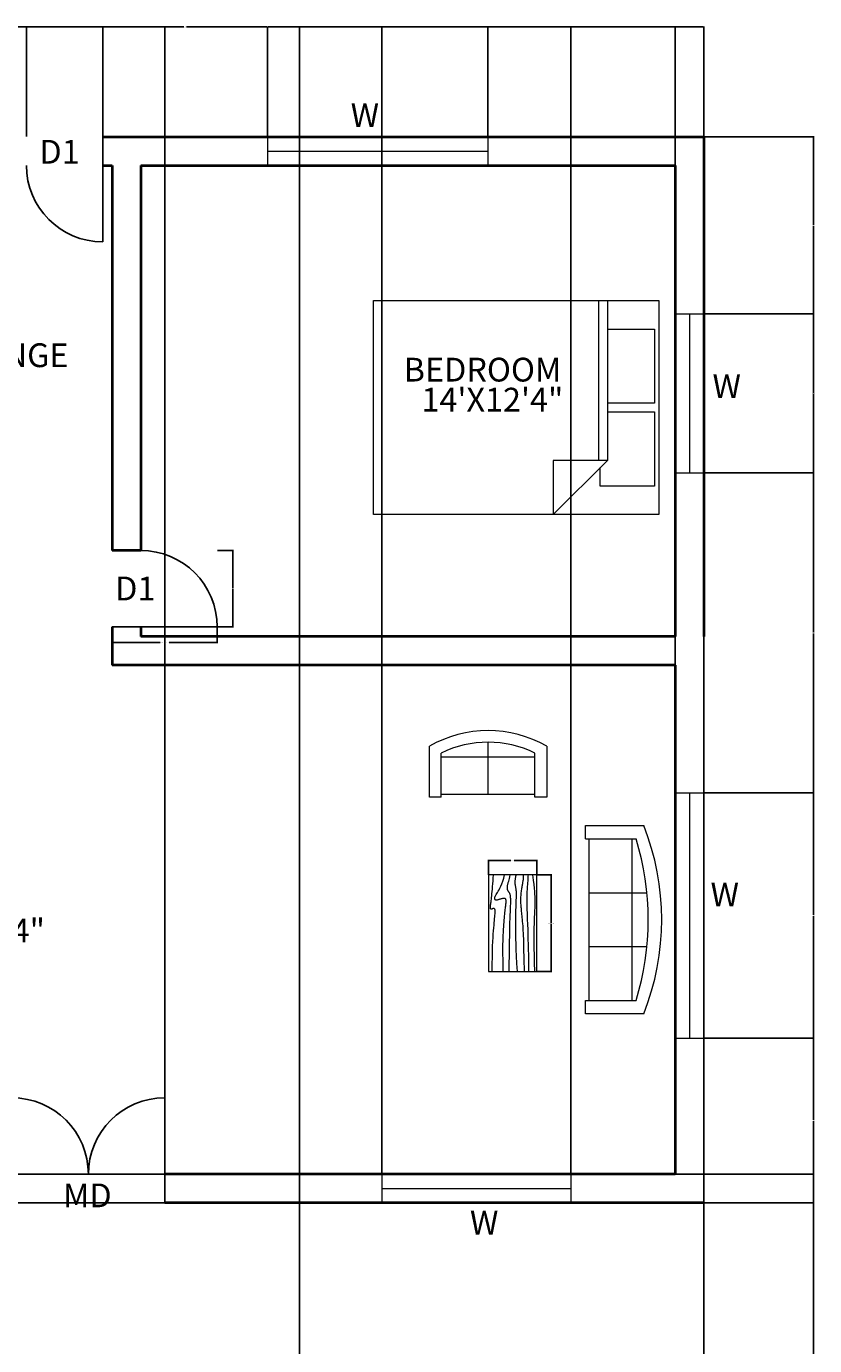
# Model space of a CAD drawing. Units: feet. Extents: x 2032 to 2763, y 1402 to 2145.
# Tile 6 of 6: x 2515 to 2763, y 1731 to 2145. Entities that reach past the tile are written whole.
import ezdxf

# ---------------------------------------------------------------- set-up
doc = ezdxf.new("R2010")
doc.units = ezdxf.units.FT
for name, color, linetype, lineweight in [('A-ANNO-DIMS', 2, 'Continuous', 18), ('A-ANNO-TEXT', 7, 'Continuous', 18), ('A-AREA-IDEN', 7, 'Continuous', 25), ('A-DOOR', 3, 'Continuous', 25), ('A-FLOR', 7, 'Continuous', 25), ('A-FURN', 8, 'Continuous', 18), ('A-GLAZ', 4, 'Continuous', 18), ('A-WALL', 7, 'Continuous', 40), ('C-PROP', 8, 'Continuous', 25)]:
    doc.layers.add(name, color=color, linetype=linetype, lineweight=lineweight)
doc.styles.get("Standard").update_dxf_attribs({"font": 'arial.ttf'})
doc.dimstyles.get("Standard").update_dxf_attribs({"dimtxt": 0.18, "dimasz": 0.18, "dimexe": 0.18, "dimexo": 0.0625, "dimgap": 0.09, "dimtad": 0, "dimtih": 1, "dimtoh": 1, "dimdec": 4, "dimzin": 0, "dimdsep": 46, "dimtxsty": 'Standard', "dimcen": 0.09, "dimadec": 0, "dimazin": 0, "dimtfac": 1, "dimtdec": 4, "dimtofl": 0, "dimtmove": 0, "dimatfit": 3, "dimfxl": 1, "dimtolj": 1, "dimtzin": 0, "dimarcsym": 0})

# ---------------------------------------------------------------- blocks, each defined once
blk = doc.blocks.new('Bed - Queen')
for p, q in [((0, -80.00003), (0, 0)), ((0, 0), (59.99999, 0)), ((59.99999, 0), (59.99999, -80.00003)), ((7.99999, -1.2), (28.79998, -1.2)), ((7.99999, -14.4), (7.99999, -1.2)), ((28.79998, -1.2), (28.79998, -14.4)), ((31.19999, -1.2), (51.99999, -1.2)), ((31.19999, -14.4), (31.19999, -1.2)), ((51.99999, -1.2), (51.99999, -16.4)), ((0, -14.4), (44.8, -14.4)), ((59.99999, -29.6), (44.8, -14.4)), ((44.8, -14.4), (44.8, -29.6)), ((44.8, -16.8), (0, -16.8)), ((51.99999, -16.4), (46.79936, -16.4)), ((44.8, -29.6), (59.99999, -29.6)), ((59.99999, -80.00003), (0, -80.00003))]:
    blk.add_line(p, q)
blk = doc.blocks.new('Sofa - Roundback 7 ft.')
for p, q in [((-36.000027, -34), (-36.000027, -11.4696)), ((-12.00002, -32.4421), (-12.00003, -6.5971)), ((11.99997, -32.4421), (11.99998, -6.5971)), ((35.99998, -34), (35.99998, -11.4696)), ((-35.999844, -13.3819), (35.9998, -13.3819)), ((-36.000027, -32.4421), (35.99998, -32.4421))]:
    blk.add_line(p, q)
for points in [[(-36.000027, -34), (-42.000027, -34), (-42.000027, -8)], [(41.99998, -8), (41.99998, -34), (35.99998, -34)]]:
    blk.add_lwpolyline(points)
for centre, radius, start, end in [((0, -114.25), 114.25, 68.43141, 111.5686), ((-0.00001, -127.1968), 121.1968, 72.72033, 107.2797)]:
    blk.add_arc(centre, radius, start, end)
blk = doc.blocks.new('Sofa - Roundback Loveseat 5 ft.')
for p, q in [((0, -32.44198), (0, -5.99998)), ((-24, -33.99998), (-24, -11.46958)), ((-23.9998, -13.38178), (23.99986, -13.38178)), ((24.00004, -33.99998), (24.00004, -11.46958)), ((-24, -32.44198), (24.00004, -32.44198))]:
    blk.add_line(p, q)
for points in [[(-24, -33.99998), (-30, -33.99998), (-30, -7.99998)], [(30.00004, -7.99998), (30.00004, -33.99998), (24.00004, -33.99998)]]:
    blk.add_lwpolyline(points)
for centre, radius, start, end in [((0, -60.24998), 60.24998, 60.13715, 119.8628), ((0, -61.38438), 55.38444, 64.32083, 115.6792)]:
    blk.add_arc(centre, radius, start, end)
blk = doc.blocks.new('Table - Rectangular Woodgrain 60 x 30 in.')
for p, q in [((0, 0), (0, -30)), ((60, 0), (0, 0)), ((60, -30), (60, 0)), ((0, -30), (60, -30))]:
    blk.add_line(p, q)
for points in [[(0, -2.4), (4.8155, -2.418), (9.0302, -2.4688), (12.709, -2.5477), (15.9167, -2.65), (18.7181, -2.7711), (21.1781, -2.9063), (23.3616, -3.0508), (25.3333, -3.2), (27.1477, -3.3495), (28.8172, -3.4958), (30.3437, -3.636), (31.7291, -3.7667), (32.9756, -3.8849), (34.0849, -3.9875), (35.059, -4.0714), (35.9, -4.1334), (36.6114, -4.1711), (37.2041, -4.1854), (37.6906, -4.1779), (38.0833, -4.15), (38.3948, -4.1034), (38.6375, -4.0396), (38.8239, -3.9602), (38.9666, -3.8667), (39.0764, -3.7608), (39.1573, -3.6448), (39.2116, -3.521), (39.2416, -3.3917), (39.2498, -3.2593), (39.2385, -3.1261), (39.21, -2.9944), (39.1666, -2.8667), (39.111, -2.7447), (39.0468, -2.6281), (38.978, -2.5163), (38.9083, -2.4083), (38.8418, -2.3035), (38.7823, -2.201), (38.7337, -2.1001), (38.7, -2), (38.6844, -1.9003), (38.6875, -1.8021), (38.7094, -1.707), (38.75, -1.6167), (38.8094, -1.5326), (38.8875, -1.4563), (38.9844, -1.3893), (39.1, -1.3333), (39.2351, -1.2896), (39.3937, -1.2583), (39.5804, -1.2396), (39.8, -1.2333), (40.057, -1.2396), (40.3562, -1.2583), (40.7023, -1.2896), (41.1, -1.3333), (41.5547, -1.3895), (42.0755, -1.4573), (42.6721, -1.5361), (43.3542, -1.625), (44.1316, -1.7233), (45.014, -1.8302), (46.0114, -1.9449), (47.1333, -2.0667), (48.3862, -2.1947), (49.7625, -2.3281), (51.2513, -2.4663), (52.8416, -2.6083), (54.5226, -2.7535), (56.2833, -2.9011), (58.1127, -3.0501), (60, -3.2)], [(0, -9.2), (6.5759, -9.0858), (11.9385, -9.0365), (16.2527, -9.0418), (19.6833, -9.0917), (22.3952, -9.1759), (24.5531, -9.2844), (26.322, -9.4069), (27.8666, -9.5333), (29.3241, -9.6553), (30.7203, -9.7719), (32.0532, -9.8837), (33.3208, -9.9917), (34.5213, -10.0965), (35.6526, -10.199), (36.7128, -10.2999), (37.7, -10.4), (38.6129, -10.4996), (39.4531, -10.5969), (40.223, -10.6895), (40.925, -10.775), (41.5613, -10.8512), (42.1344, -10.9156), (42.6465, -10.966), (43.1, -11), (43.4976, -11.0158), (43.8437, -11.0136), (44.143, -10.9942), (44.4, -10.9583), (44.6195, -10.9069), (44.8062, -10.8406), (44.9648, -10.7603), (45.1, -10.6667), (45.2155, -10.5598), (45.3114, -10.4365), (45.3871, -10.2929), (45.4416, -10.125), (45.4743, -9.929), (45.4844, -9.7011), (45.4709, -9.4371), (45.4333, -9.1333), (45.3716, -8.7883), (45.2896, -8.4104), (45.1919, -8.0107), (45.0833, -7.6), (44.9685, -7.1893), (44.8521, -6.7896), (44.7388, -6.4117), (44.6333, -6.0667), (44.54, -5.7628), (44.4614, -5.4979), (44.4001, -5.2675), (44.3583, -5.0667), (44.3384, -4.8909), (44.3427, -4.7354), (44.3736, -4.5956), (44.4333, -4.4667), (44.5236, -4.3453), (44.6427, -4.2333), (44.7884, -4.1339), (44.9583, -4.05), (45.1501, -3.9849), (45.3614, -3.9417), (45.59, -3.9234), (45.8333, -3.9333), (46.0915, -3.9749), (46.3734, -4.0531), (46.6906, -4.1736), (47.0542, -4.3417), (47.4756, -4.5629), (47.9661, -4.8427), (48.5372, -5.1866), (49.2, -5.6), (49.9676, -6.0844), (50.8594, -6.625), (51.8965, -7.2031), (53.1, -7.8), (54.491, -8.3969), (56.0906, -8.975), (57.9199, -9.5156), (60, -10)], [(0, -12.8), (5.1847, -12.9322), (9.6213, -13.0323), (13.3963, -13.1059), (16.5958, -13.1583), (19.3063, -13.1952), (21.614, -13.2219), (23.6054, -13.2439), (25.3666, -13.2667), (26.9728, -13.2947), (28.4531, -13.3281), (29.8256, -13.3663), (31.1083, -13.4083), (32.3191, -13.4535), (33.476, -13.501), (34.597, -13.5501), (35.7, -13.6), (36.7984, -13.6497), (37.8875, -13.6979), (38.9578, -13.743), (40, -13.7833), (41.0047, -13.8174), (41.9625, -13.8438), (42.864, -13.8607), (43.7, -13.8667), (44.4631, -13.8604), (45.1552, -13.8417), (45.7801, -13.8104), (46.3416, -13.7667), (46.8439, -13.7104), (47.2906, -13.6417), (47.6858, -13.5604), (48.0333, -13.4667), (48.3375, -13.3608), (48.6042, -13.2448), (48.8396, -13.121), (49.05, -12.9917), (49.2417, -12.8593), (49.4208, -12.7261), (49.5937, -12.5944), (49.7667, -12.4667), (49.9452, -12.3451), (50.1323, -12.2313), (50.3303, -12.1268), (50.5416, -12.0333), (50.7686, -11.9524), (51.0135, -11.8854), (51.2788, -11.8341), (51.5666, -11.8), (51.8785, -11.7843), (52.2116, -11.7865), (52.562, -11.8059), (52.926, -11.8417), (53.2998, -11.8931), (53.6795, -11.9594), (54.0614, -12.0397), (54.4416, -12.1333), (54.8223, -12.2401), (55.2293, -12.3625), (55.6942, -12.5037), (56.2489, -12.6667), (56.9251, -12.8547), (57.7545, -13.0708), (58.7689, -13.3182), (60, -13.6)], [(0, -18), (5.124, -17.7273), (9.6609, -17.5057), (13.6705, -17.3303), (17.2125, -17.1958), (20.3467, -17.0973), (23.1328, -17.0297), (25.6307, -16.9878), (27.9, -16.9667), (29.9928, -16.9617), (31.9302, -16.9703), (33.7254, -16.9907), (35.3917, -17.0208), (36.9423, -17.0588), (38.3906, -17.1026), (39.7499, -17.1503), (41.0333, -17.2), (42.2519, -17.2496), (43.4073, -17.2969), (44.4986, -17.3395), (45.525, -17.375), (46.4858, -17.4012), (47.3802, -17.4156), (48.2074, -17.416), (48.9667, -17.4), (49.6583, -17.3662), (50.2872, -17.3167), (50.8595, -17.2547), (51.3812, -17.1833), (51.8584, -17.1057), (52.2971, -17.025), (52.7034, -16.9443), (53.0833, -16.8667), (53.443, -16.7951), (53.789, -16.7313), (54.128, -16.6768), (54.4666, -16.6334), (54.8115, -16.6024), (55.1693, -16.5854), (55.5465, -16.5841), (55.95, -16.6), (56.3828, -16.6337), (56.8346, -16.6823), (57.2915, -16.7418), (57.7396, -16.8084), (58.165, -16.878), (58.5539, -16.9469), (58.8924, -17.0111), (59.1666, -17.0667), (59.3679, -17.1107), (59.5078, -17.1438), (59.6032, -17.1675), (59.6708, -17.1833), (59.7275, -17.193), (59.7901, -17.1979), (59.8753, -17.1998), (60, -17.2)], [(0, -22.4), (8.0098, -22.2501), (14.4094, -22.1011), (19.4168, -21.9535), (23.25, -21.8083), (26.1269, -21.6663), (28.2656, -21.5281), (29.884, -21.3947), (31.2, -21.2667), (32.3967, -21.1448), (33.5172, -21.0292), (34.5697, -20.9198), (35.5625, -20.8167), (36.5037, -20.7198), (37.4015, -20.6292), (38.2642, -20.5448), (39.1, -20.4667), (39.9164, -20.3951), (40.7187, -20.3313), (41.5117, -20.2768), (42.3, -20.2333), (43.0883, -20.2024), (43.8812, -20.1854), (44.6836, -20.1841), (45.5, -20.2), (46.3328, -20.234), (47.1747, -20.2844), (48.0163, -20.3488), (48.8479, -20.425), (49.66, -20.5106), (50.4429, -20.6031), (51.1872, -20.7004), (51.8833, -20.8), (52.5246, -20.8999), (53.1166, -20.9995), (53.6681, -21.0983), (54.1875, -21.1958), (54.6834, -21.2919), (55.1646, -21.3859), (55.6394, -21.4777), (56.1167, -21.5667), (56.6028, -21.6515), (57.0961, -21.7266), (57.5929, -21.7852), (58.0896, -21.8208), (58.5823, -21.8268), (59.0674, -21.7964), (59.5412, -21.723), (60, -21.6)], [(0, -25.2), (8.6355, -25.0504), (15.7026, -24.9031), (21.4049, -24.7606), (25.9458, -24.625), (29.529, -24.4988), (32.3578, -24.3844), (34.6359, -24.284), (36.5667, -24.2), (38.3213, -24.1341), (39.9417, -24.0854), (41.437, -24.0523), (42.8167, -24.0333), (44.0901, -24.0268), (45.2667, -24.0313), (46.3557, -24.0451), (47.3667, -24.0667), (48.309, -24.0947), (49.1928, -24.1287), (50.0284, -24.168), (50.826, -24.2125), (51.5959, -24.2617), (52.3483, -24.3151), (53.0935, -24.3725), (53.8417, -24.4334), (54.6009, -24.497), (55.3699, -24.561), (56.1454, -24.6226), (56.9239, -24.6792), (57.7021, -24.7279), (58.4764, -24.7662), (59.2435, -24.7911), (60, -24.8)], [(0, -28.8), (5.6867, -28.6681), (10.45, -28.5698), (14.407, -28.5012), (17.675, -28.4584), (20.3711, -28.4374), (22.6125, -28.4344), (24.5164, -28.4455), (26.2, -28.4667), (27.762, -28.4947), (29.2276, -28.5281), (30.6033, -28.5663), (31.8958, -28.6084), (33.1118, -28.6535), (34.2578, -28.7011), (35.3405, -28.7501), (36.3666, -28.8), (37.3443, -28.8497), (38.288, -28.8974), (39.2137, -28.9412), (40.1375, -28.9792), (41.0753, -29.0093), (42.0432, -29.0297), (43.0572, -29.0384), (44.1333, -29.0333), (45.2936, -29.0114), (46.5843, -28.9641), (48.0579, -28.8816), (49.7666, -28.7542), (51.7629, -28.5721), (54.0989, -28.3255), (56.8272, -28.0048), (60, -27.6)]]:
    blk.add_lwpolyline(points)
blk = doc.blocks.new('DOOR-SWING-24')
blk.add_line((33, 0), (0, 0))
blk.add_arc((9, 0), 24, 0, 90)
blk = doc.blocks.new('*D11')
at = {"layer": 'A-ANNO-DIMS', "color": 0, "lineweight": -2, "transparency": 16777216}
for p, q in [((2542.31, 1956.55), (2542.31, 1951.48)), ((2575.31, 1956.55), (2575.31, 1951.48)), ((2542.49, 1951.66), (2557.38, 1951.66)), ((2575.13, 1951.66), (2560.25, 1951.66))]:
    blk.add_line(p, q, dxfattribs=at)
at = {"layer": 'A-ANNO-DIMS', "color": 0, "transparency": 16777216}
for points in [[(2542.49, 1951.69), (2542.49, 1951.63), (2542.31, 1951.66)], [(2575.13, 1951.69), (2575.13, 1951.63), (2575.31, 1951.66)]]:
    blk.add_solid(points, dxfattribs=at)
at = {"layer": 'Defpoints', "color": 0, "transparency": 16777216}
for p in [(2542.31, 1956.61), (2575.31, 1956.61), (2575.31, 1951.66)]:
    blk.add_point(p, dxfattribs=at)
at = {"layer": 'A-ANNO-DIMS', "color": 0, "transparency": 16777216, "insert": (2558.81, 1951.66), "char_height": 0.18, "attachment_point": 5}
blk.add_mtext('\\A1;SINGLE DOOR 33 TYP.', dxfattribs=at)
blk = doc.blocks.new('*D12')
at = {"layer": 'A-ANNO-DIMS', "color": 0, "lineweight": -2, "transparency": 16777216}
for p, q in [((2575.38, 1980.61), (2580.44, 1980.61)), ((2580.26, 1980.43), (2580.26, 1968.79)), ((2580.26, 1956.79), (2580.26, 1968.43)), ((2575.38, 1956.61), (2580.44, 1956.61))]:
    blk.add_line(p, q, dxfattribs=at)
at = {"layer": 'A-ANNO-DIMS', "color": 0, "transparency": 16777216}
for points in [[(2580.23, 1980.43), (2580.29, 1980.43), (2580.26, 1980.61)], [(2580.23, 1956.79), (2580.29, 1956.79), (2580.26, 1956.61)]]:
    blk.add_solid(points, dxfattribs=at)
at = {"layer": 'Defpoints', "color": 0, "transparency": 16777216}
for p in [(2575.31, 1980.61), (2580.26, 1980.61), (2575.31, 1956.61)]:
    blk.add_point(p, dxfattribs=at)
at = {"layer": 'A-ANNO-DIMS', "color": 0, "transparency": 16777216, "insert": (2580.26, 1968.61), "char_height": 0.18, "attachment_point": 5}
blk.add_mtext('\\A1;24 TYP.', dxfattribs=at)
blk = doc.blocks.new('*D23')
at = {"layer": 'A-ANNO-DIMS', "color": 0, "lineweight": -2, "transparency": 16777216}
for p, q in [((2675.86, 1878.65), (2680.53, 1878.65)), ((2680.35, 1878.47), (2680.35, 1863.64)), ((2680.35, 1848.45), (2680.35, 1863.27)), ((2675.86, 1848.27), (2680.53, 1848.27))]:
    blk.add_line(p, q, dxfattribs=at)
at = {"layer": 'A-ANNO-DIMS', "color": 0, "transparency": 16777216}
for points in [[(2680.32, 1878.47), (2680.38, 1878.47), (2680.35, 1878.65)], [(2680.32, 1848.45), (2680.38, 1848.45), (2680.35, 1848.27)]]:
    blk.add_solid(points, dxfattribs=at)
at = {"layer": 'Defpoints', "color": 0, "transparency": 16777216}
for p in [(2675.79, 1878.65), (2680.35, 1878.65), (2675.79, 1848.27)]:
    blk.add_point(p, dxfattribs=at)
at = {"layer": 'A-ANNO-DIMS', "color": 0, "transparency": 16777216, "insert": (2680.35, 1863.46), "char_height": 0.18, "attachment_point": 5}
blk.add_mtext('\\A1;TABLE 30 TYP.', dxfattribs=at)
blk = doc.blocks.new('*D24')
at = {"layer": 'A-ANNO-DIMS', "color": 0, "lineweight": -2, "transparency": 16777216}
for p, q in [((2660.6, 1878.71), (2660.6, 1883.38)), ((2660.78, 1883.2), (2667.68, 1883.2)), ((2675.61, 1883.2), (2668.72, 1883.2)), ((2675.79, 1878.71), (2675.79, 1883.38))]:
    blk.add_line(p, q, dxfattribs=at)
at = {"layer": 'A-ANNO-DIMS', "color": 0, "transparency": 16777216}
for points in [[(2660.78, 1883.23), (2660.78, 1883.17), (2660.6, 1883.2)], [(2675.61, 1883.23), (2675.61, 1883.17), (2675.79, 1883.2)]]:
    blk.add_solid(points, dxfattribs=at)
at = {"layer": 'Defpoints', "color": 0, "transparency": 16777216}
for p in [(2660.6, 1883.2), (2660.6, 1878.65), (2675.79, 1878.65)]:
    blk.add_point(p, dxfattribs=at)
at = {"layer": 'A-ANNO-DIMS', "color": 0, "transparency": 16777216, "insert": (2668.2, 1883.2), "char_height": 0.18, "attachment_point": 5}
blk.add_mtext('\\A1;15 TYP.', dxfattribs=at)
blk = doc.blocks.new('*D43')
at = {"layer": 'A-ANNO-DIMS', "color": 0, "lineweight": -2, "transparency": 16777216}
for p, q in [((2515.31, 2110.68), (2515.31, 2145.29)), ((2515.49, 2145.11), (2527.09, 2145.11)), ((2539.13, 2145.11), (2527.53, 2145.11)), ((2539.31, 2110.68), (2539.31, 2145.29))]:
    blk.add_line(p, q, dxfattribs=at)
at = {"layer": 'A-ANNO-DIMS', "color": 0, "transparency": 16777216}
for points in [[(2515.49, 2145.14), (2515.49, 2145.08), (2515.31, 2145.11)], [(2539.13, 2145.14), (2539.13, 2145.08), (2539.31, 2145.11)]]:
    blk.add_solid(points, dxfattribs=at)
at = {"layer": 'Defpoints', "color": 0, "transparency": 16777216}
for p in [(2539.31, 2145.11), (2515.31, 2110.61), (2539.31, 2110.61)]:
    blk.add_point(p, dxfattribs=at)
at = {"layer": 'A-ANNO-DIMS', "color": 0, "transparency": 16777216, "insert": (2527.31, 2145.11), "char_height": 0.18, "attachment_point": 5}
blk.add_mtext('\\A1;24', dxfattribs=at)
blk = doc.blocks.new('*D44')
at = {"layer": 'A-ANNO-DIMS', "color": 0, "lineweight": -2, "transparency": 16777216}
for p, q in [((2539.31, 2110.68), (2539.31, 2145.29)), ((2539.49, 2145.11), (2564.83, 2145.11)), ((2590.95, 2145.11), (2565.62, 2145.11)), ((2591.13, 2110.68), (2591.13, 2145.29))]:
    blk.add_line(p, q, dxfattribs=at)
at = {"layer": 'A-ANNO-DIMS', "color": 0, "transparency": 16777216}
for points in [[(2539.49, 2145.14), (2539.49, 2145.08), (2539.31, 2145.11)], [(2590.95, 2145.14), (2590.95, 2145.08), (2591.13, 2145.11)]]:
    blk.add_solid(points, dxfattribs=at)
at = {"layer": 'Defpoints', "color": 0, "transparency": 16777216}
for p in [(2591.13, 2145.11), (2539.31, 2110.61), (2591.13, 2110.61)]:
    blk.add_point(p, dxfattribs=at)
at = {"layer": 'A-ANNO-DIMS', "color": 0, "transparency": 16777216, "insert": (2565.22, 2145.11), "char_height": 0.18, "attachment_point": 5}
blk.add_mtext('\\A1;51.82', dxfattribs=at)
blk = doc.blocks.new('*D45')
at = {"layer": 'A-ANNO-DIMS', "color": 0, "lineweight": -2, "transparency": 16777216}
for p, q in [((2591.13, 2110.68), (2591.13, 2145.29)), ((2591.31, 2145.11), (2625.38, 2145.11)), ((2660.23, 2145.11), (2626.16, 2145.11)), ((2660.41, 2110.68), (2660.41, 2145.29))]:
    blk.add_line(p, q, dxfattribs=at)
at = {"layer": 'A-ANNO-DIMS', "color": 0, "transparency": 16777216}
for points in [[(2591.31, 2145.14), (2591.31, 2145.08), (2591.13, 2145.11)], [(2660.23, 2145.14), (2660.23, 2145.08), (2660.41, 2145.11)]]:
    blk.add_solid(points, dxfattribs=at)
at = {"layer": 'Defpoints', "color": 0, "transparency": 16777216}
for p in [(2660.41, 2145.11), (2591.13, 2110.61), (2660.41, 2110.61)]:
    blk.add_point(p, dxfattribs=at)
at = {"layer": 'A-ANNO-DIMS', "color": 0, "transparency": 16777216, "insert": (2625.77, 2145.11), "char_height": 0.18, "attachment_point": 5}
blk.add_mtext('\\A1;69.28', dxfattribs=at)
blk = doc.blocks.new('*D46')
at = {"layer": 'A-ANNO-DIMS', "color": 0, "lineweight": -2, "transparency": 16777216}
for p, q in [((2660.41, 2110.68), (2660.41, 2145.29)), ((2660.59, 2145.11), (2694.04, 2145.11)), ((2728.13, 2145.11), (2694.69, 2145.11)), ((2728.31, 2110.68), (2728.31, 2145.29))]:
    blk.add_line(p, q, dxfattribs=at)
at = {"layer": 'A-ANNO-DIMS', "color": 0, "transparency": 16777216}
for points in [[(2660.59, 2145.14), (2660.59, 2145.08), (2660.41, 2145.11)], [(2728.13, 2145.14), (2728.13, 2145.08), (2728.31, 2145.11)]]:
    blk.add_solid(points, dxfattribs=at)
at = {"layer": 'Defpoints', "color": 0, "transparency": 16777216}
for p in [(2728.31, 2145.11), (2660.41, 2110.61), (2728.31, 2110.61)]:
    blk.add_point(p, dxfattribs=at)
at = {"layer": 'A-ANNO-DIMS', "color": 0, "transparency": 16777216, "insert": (2694.36, 2145.11), "char_height": 0.18, "attachment_point": 5}
blk.add_mtext('\\A1;67.9', dxfattribs=at)
blk = doc.blocks.new('*D48')
at = {"layer": 'A-ANNO-DIMS', "color": 0, "lineweight": -2, "transparency": 16777216}
for p, q in [((2601.22, 1775.61), (2762.99, 1775.61)), ((2762.81, 1775.43), (2762.81, 1636.29)), ((2762.81, 1496.79), (2762.81, 1635.93)), ((2601.22, 1496.61), (2762.99, 1496.61))]:
    blk.add_line(p, q, dxfattribs=at)
at = {"layer": 'A-ANNO-DIMS', "color": 0, "transparency": 16777216}
for points in [[(2762.78, 1775.43), (2762.84, 1775.43), (2762.81, 1775.61)], [(2762.78, 1496.79), (2762.84, 1496.79), (2762.81, 1496.61)]]:
    blk.add_solid(points, dxfattribs=at)
at = {"layer": 'Defpoints', "color": 0, "transparency": 16777216}
for p in [(2601.16, 1775.61), (2762.81, 1775.61), (2601.16, 1496.61)]:
    blk.add_point(p, dxfattribs=at)
at = {"layer": 'A-ANNO-DIMS', "color": 0, "transparency": 16777216, "insert": (2762.81, 1636.11), "char_height": 0.18, "attachment_point": 5}
blk.add_mtext('\\A1;279', dxfattribs=at)
blk = doc.blocks.new('*D62')
at = {"layer": 'A-ANNO-DIMS', "color": 0, "lineweight": -2, "transparency": 16777216}
for p, q in [((2728.38, 1827.33), (2762.99, 1827.33)), ((2762.81, 1827.15), (2762.81, 1801.66)), ((2762.81, 1775.79), (2762.81, 1801.29)), ((2728.38, 1775.61), (2762.99, 1775.61))]:
    blk.add_line(p, q, dxfattribs=at)
at = {"layer": 'A-ANNO-DIMS', "color": 0, "transparency": 16777216}
for points in [[(2762.78, 1827.15), (2762.84, 1827.15), (2762.81, 1827.33)], [(2762.78, 1775.79), (2762.84, 1775.79), (2762.81, 1775.61)]]:
    blk.add_solid(points, dxfattribs=at)
at = {"layer": 'Defpoints', "color": 0, "transparency": 16777216}
for p in [(2728.31, 1827.33), (2762.81, 1827.33), (2728.31, 1775.61)]:
    blk.add_point(p, dxfattribs=at)
at = {"layer": 'A-ANNO-DIMS', "color": 0, "transparency": 16777216, "insert": (2762.81, 1801.47), "char_height": 0.18, "attachment_point": 5}
blk.add_mtext('\\A1;51.72', dxfattribs=at)
blk = doc.blocks.new('*D63')
at = {"layer": 'A-ANNO-DIMS', "color": 0, "lineweight": -2, "transparency": 16777216}
for p, q in [((2728.38, 1904.45), (2762.99, 1904.45)), ((2762.81, 1904.27), (2762.81, 1866.07)), ((2762.81, 1827.51), (2762.81, 1865.71)), ((2728.38, 1827.33), (2762.99, 1827.33))]:
    blk.add_line(p, q, dxfattribs=at)
at = {"layer": 'A-ANNO-DIMS', "color": 0, "transparency": 16777216}
for points in [[(2762.78, 1904.27), (2762.84, 1904.27), (2762.81, 1904.45)], [(2762.78, 1827.51), (2762.84, 1827.51), (2762.81, 1827.33)]]:
    blk.add_solid(points, dxfattribs=at)
at = {"layer": 'Defpoints', "color": 0, "transparency": 16777216}
for p in [(2728.31, 1904.45), (2762.81, 1904.45), (2728.31, 1827.33)]:
    blk.add_point(p, dxfattribs=at)
at = {"layer": 'A-ANNO-DIMS', "color": 0, "transparency": 16777216, "insert": (2762.81, 1865.89), "char_height": 0.18, "attachment_point": 5}
blk.add_mtext('\\A1;77.11', dxfattribs=at)
blk = doc.blocks.new('*D64')
at = {"layer": 'A-ANNO-DIMS', "color": 0, "lineweight": -2, "transparency": 16777216}
for p, q in [((2728.38, 2004.99), (2762.99, 2004.99)), ((2762.81, 2004.81), (2762.81, 1954.9)), ((2762.81, 1904.63), (2762.81, 1954.54)), ((2728.38, 1904.45), (2762.99, 1904.45))]:
    blk.add_line(p, q, dxfattribs=at)
at = {"layer": 'A-ANNO-DIMS', "color": 0, "transparency": 16777216}
for points in [[(2762.78, 2004.81), (2762.84, 2004.81), (2762.81, 2004.99)], [(2762.78, 1904.63), (2762.84, 1904.63), (2762.81, 1904.45)]]:
    blk.add_solid(points, dxfattribs=at)
at = {"layer": 'Defpoints', "color": 0, "transparency": 16777216}
for p in [(2728.31, 2004.99), (2762.81, 2004.99), (2728.31, 1904.45)]:
    blk.add_point(p, dxfattribs=at)
at = {"layer": 'A-ANNO-DIMS', "color": 0, "transparency": 16777216, "insert": (2762.81, 1954.72), "char_height": 0.18, "attachment_point": 5}
blk.add_mtext('\\A1;100.54', dxfattribs=at)
blk = doc.blocks.new('*D65')
at = {"layer": 'A-ANNO-DIMS', "color": 0, "lineweight": -2, "transparency": 16777216}
for p, q in [((2728.38, 2054.95), (2762.99, 2054.95)), ((2762.81, 2054.77), (2762.81, 2030.15)), ((2762.81, 2005.17), (2762.81, 2029.79)), ((2728.38, 2004.99), (2762.99, 2004.99))]:
    blk.add_line(p, q, dxfattribs=at)
at = {"layer": 'A-ANNO-DIMS', "color": 0, "transparency": 16777216}
for points in [[(2762.78, 2054.77), (2762.84, 2054.77), (2762.81, 2054.95)], [(2762.78, 2005.17), (2762.84, 2005.17), (2762.81, 2004.99)]]:
    blk.add_solid(points, dxfattribs=at)
at = {"layer": 'Defpoints', "color": 0, "transparency": 16777216}
for p in [(2728.31, 2054.95), (2762.81, 2054.95), (2728.31, 2004.99)]:
    blk.add_point(p, dxfattribs=at)
at = {"layer": 'A-ANNO-DIMS', "color": 0, "transparency": 16777216, "insert": (2762.81, 2029.97), "char_height": 0.18, "attachment_point": 5}
blk.add_mtext('\\A1;49.97', dxfattribs=at)
blk = doc.blocks.new('*D66')
at = {"layer": 'A-ANNO-DIMS', "color": 0, "lineweight": -2, "transparency": 16777216}
for p, q in [((2728.38, 2110.61), (2762.99, 2110.61)), ((2762.81, 2110.43), (2762.81, 2082.97)), ((2762.81, 2055.13), (2762.81, 2082.6)), ((2728.38, 2054.95), (2762.99, 2054.95))]:
    blk.add_line(p, q, dxfattribs=at)
at = {"layer": 'A-ANNO-DIMS', "color": 0, "transparency": 16777216}
for points in [[(2762.78, 2110.43), (2762.84, 2110.43), (2762.81, 2110.61)], [(2762.78, 2055.13), (2762.84, 2055.13), (2762.81, 2054.95)]]:
    blk.add_solid(points, dxfattribs=at)
at = {"layer": 'Defpoints', "color": 0, "transparency": 16777216}
for p in [(2728.31, 2110.61), (2762.81, 2110.61), (2728.31, 2054.95)]:
    blk.add_point(p, dxfattribs=at)
at = {"layer": 'A-ANNO-DIMS', "color": 0, "transparency": 16777216, "insert": (2762.81, 2082.78), "char_height": 0.18, "attachment_point": 5}
blk.add_mtext('\\A1;55.66', dxfattribs=at)
blk = doc.blocks.new('*D74')
at = {"layer": 'A-ANNO-DIMS', "color": 0, "lineweight": -2, "transparency": 16777216}
for p, q in [((2510.81, 1775.68), (2510.81, 2145.29)), ((2510.99, 2145.11), (2534.59, 2145.11)), ((2558.63, 2145.11), (2535.04, 2145.11)), ((2558.81, 1775.68), (2558.81, 2145.29))]:
    blk.add_line(p, q, dxfattribs=at)
at = {"layer": 'A-ANNO-DIMS', "color": 0, "transparency": 16777216}
for points in [[(2510.99, 2145.14), (2510.99, 2145.08), (2510.81, 2145.11)], [(2558.63, 2145.14), (2558.63, 2145.08), (2558.81, 2145.11)]]:
    blk.add_solid(points, dxfattribs=at)
at = {"layer": 'Defpoints', "color": 0, "transparency": 16777216}
for p in [(2558.81, 2145.11), (2510.81, 1775.61), (2558.81, 1775.61)]:
    blk.add_point(p, dxfattribs=at)
at = {"layer": 'A-ANNO-DIMS', "color": 0, "transparency": 16777216, "insert": (2534.81, 2145.11), "char_height": 0.18, "attachment_point": 5}
blk.add_mtext('\\A1;48', dxfattribs=at)
blk = doc.blocks.new('*D75')
at = {"layer": 'A-ANNO-DIMS', "color": 0, "lineweight": -2, "transparency": 16777216}
for p, q in [((2601.16, 1775.68), (2601.16, 2145.29)), ((2601.34, 2145.11), (2613.67, 2145.11)), ((2626.92, 2145.11), (2614.6, 2145.11)), ((2627.1, 1784.68), (2627.1, 2145.29))]:
    blk.add_line(p, q, dxfattribs=at)
at = {"layer": 'A-ANNO-DIMS', "color": 0, "transparency": 16777216}
for points in [[(2601.34, 2145.14), (2601.34, 2145.08), (2601.16, 2145.11)], [(2626.92, 2145.14), (2626.92, 2145.08), (2627.1, 2145.11)]]:
    blk.add_solid(points, dxfattribs=at)
at = {"layer": 'Defpoints', "color": 0, "transparency": 16777216}
for p in [(2627.1, 2145.11), (2627.1, 1784.61), (2601.16, 1775.61)]:
    blk.add_point(p, dxfattribs=at)
at = {"layer": 'A-ANNO-DIMS', "color": 0, "transparency": 16777216, "insert": (2614.13, 2145.11), "char_height": 0.18, "attachment_point": 5}
blk.add_mtext('\\A1;25.946', dxfattribs=at)
blk = doc.blocks.new('*D76')
at = {"layer": 'A-ANNO-DIMS', "color": 0, "lineweight": -2, "transparency": 16777216}
for p, q in [((2627.1, 1784.68), (2627.1, 2145.29)), ((2627.28, 2145.11), (2656.43, 2145.11)), ((2686.37, 2145.11), (2657.22, 2145.11)), ((2686.55, 1784.68), (2686.55, 2145.29))]:
    blk.add_line(p, q, dxfattribs=at)
at = {"layer": 'A-ANNO-DIMS', "color": 0, "transparency": 16777216}
for points in [[(2627.28, 2145.14), (2627.28, 2145.08), (2627.1, 2145.11)], [(2686.37, 2145.14), (2686.37, 2145.08), (2686.55, 2145.11)]]:
    blk.add_solid(points, dxfattribs=at)
at = {"layer": 'Defpoints', "color": 0, "transparency": 16777216}
for p in [(2686.55, 2145.11), (2627.1, 1784.61), (2686.55, 1784.61)]:
    blk.add_point(p, dxfattribs=at)
at = {"layer": 'A-ANNO-DIMS', "color": 0, "transparency": 16777216, "insert": (2656.83, 2145.11), "char_height": 0.18, "attachment_point": 5}
blk.add_mtext('\\A1;59.45', dxfattribs=at)
blk = doc.blocks.new('*D77')
at = {"layer": 'A-ANNO-DIMS', "color": 0, "lineweight": -2, "transparency": 16777216}
for p, q in [((2686.55, 1784.68), (2686.55, 2145.29)), ((2686.73, 2145.11), (2702.54, 2145.11)), ((2719.13, 2145.11), (2703.33, 2145.11)), ((2719.31, 1784.68), (2719.31, 2145.29))]:
    blk.add_line(p, q, dxfattribs=at)
at = {"layer": 'A-ANNO-DIMS', "color": 0, "transparency": 16777216}
for points in [[(2686.73, 2145.14), (2686.73, 2145.08), (2686.55, 2145.11)], [(2719.13, 2145.14), (2719.13, 2145.08), (2719.31, 2145.11)]]:
    blk.add_solid(points, dxfattribs=at)
at = {"layer": 'Defpoints', "color": 0, "transparency": 16777216}
for p in [(2719.31, 2145.11), (2686.55, 1784.61), (2719.31, 1784.61)]:
    blk.add_point(p, dxfattribs=at)
at = {"layer": 'A-ANNO-DIMS', "color": 0, "transparency": 16777216, "insert": (2702.93, 2145.11), "char_height": 0.18, "attachment_point": 5}
blk.add_mtext('\\A1;32.76', dxfattribs=at)
blk = doc.blocks.new('*D82')
at = {"layer": 'A-ANNO-DIMS', "color": 0, "lineweight": -2, "transparency": 16777216}
for p, q in [((2293.38, 1784.61), (2762.99, 1784.61)), ((2762.81, 1784.43), (2762.81, 1780.29)), ((2762.81, 1775.79), (2762.81, 1779.93)), ((2293.38, 1775.61), (2762.99, 1775.61))]:
    blk.add_line(p, q, dxfattribs=at)
at = {"layer": 'A-ANNO-DIMS', "color": 0, "transparency": 16777216}
for points in [[(2762.78, 1784.43), (2762.84, 1784.43), (2762.81, 1784.61)], [(2762.78, 1775.79), (2762.84, 1775.79), (2762.81, 1775.61)]]:
    blk.add_solid(points, dxfattribs=at)
at = {"layer": 'Defpoints', "color": 0, "transparency": 16777216}
for p in [(2293.31, 1784.61), (2762.81, 1784.61), (2293.31, 1775.61)]:
    blk.add_point(p, dxfattribs=at)
at = {"layer": 'A-ANNO-DIMS', "color": 0, "transparency": 16777216, "insert": (2762.81, 1780.11), "char_height": 0.18, "attachment_point": 5}
blk.add_mtext('\\A1;9', dxfattribs=at)

msp = doc.modelspace()

# ---------------------------------------------------------------- linework, layer by layer
at = {"layer": 'A-FLOR'}
msp.add_line((2601.1579, 1496.6131), (2601.1579, 1775.6131), dxfattribs=at)
at = {"layer": 'A-GLAZ'}
for p, q in [((2591.1312, 2110.6131), (2591.1312, 2101.6131)), ((2660.4084, 2110.6131), (2660.4084, 2101.6131)), ((2591.1312, 2106.1131), (2660.4084, 2106.1131)), ((2719.3136, 2054.955), (2728.3136, 2054.955)), ((2723.8136, 2054.955), (2723.8136, 2004.9896)), ((2719.3136, 2004.9896), (2728.3136, 2004.9896)), ((2719.3136, 1904.446), (2728.3136, 1904.446)), ((2723.8136, 1904.446), (2723.8136, 1827.3345)), ((2719.3136, 1827.3345), (2728.3136, 1827.3345)), ((2627.1044, 1784.6131), (2627.1044, 1775.6131)), ((2686.5524, 1784.6131), (2686.5524, 1775.6131)), ((2627.1044, 1780.1131), (2686.5524, 1780.1131))]:
    msp.add_line(p, q, dxfattribs=at)
at = {"layer": 'A-WALL'}
for p, q in [((2539.3136, 2110.6131), (2728.3136, 2110.6131)), ((2539.3136, 2110.6131), (2542.3136, 2110.6131)), ((2728.3136, 2110.6131), (2728.3136, 1953.6131)), ((2539.3136, 2101.6131), (2542.3136, 2101.6131)), ((2542.3136, 2101.6131), (2542.3136, 1980.6131)), ((2551.3136, 2101.6131), (2551.3136, 1980.6131)), ((2551.3136, 2101.6131), (2719.3136, 2101.6131)), ((2719.3136, 2101.6131), (2719.3136, 1953.6131)), ((2551.3136, 1980.6131), (2542.3136, 1980.6131)), ((2542.3136, 1956.6131), (2542.3136, 1944.6131)), ((2551.3136, 1956.6131), (2551.3136, 1953.6131)), ((2719.3136, 1953.6131), (2551.3136, 1953.6131)), ((2719.3136, 1944.6131), (2542.3136, 1944.6131)), ((2719.3136, 1944.6131), (2551.3136, 1944.6131)), ((2719.3136, 1944.6131), (2719.3136, 1784.6131)), ((2719.3136, 1784.6131), (2558.8136, 1784.6131)), ((2728.3136, 1775.6131), (2558.8136, 1775.6131))]:
    msp.add_line(p, q, dxfattribs=at)
at = {"layer": 'C-PROP'}
msp.add_line((2728.3136, 2110.6131), (2728.3136, 1496.6131), dxfattribs=at)

# ---------------------------------------------------------------- block references
at = {"layer": 'A-DOOR', "extrusion": (0, 0, -1), "zscale": -1}
for p, rotation in [((-2539.3137, 2110.6127), 269.9999999999995), ((-2510.8136, 1775.6134), 90.0000000000006)]:
    msp.add_blockref('DOOR-SWING-24', p, dxfattribs=dict(at, rotation=rotation))
at = {"layer": 'A-DOOR'}
msp.add_blockref('DOOR-SWING-24', (2542.314, 1956.613), dxfattribs=at)
at = {"layer": 'A-DOOR', "rotation": 90.00000000000011}
msp.add_blockref('DOOR-SWING-24', (2558.8137, 1775.6134), dxfattribs=at)
at = {"layer": 'A-FURN'}
for name, p, xscale, yscale, zscale, rotation in [('Bed - Queen', (2714.1847, 2059.1681), 1.121589901058193, 1.121589901058193, 1.121589901058193, 270), ('Sofa - Roundback 7 ft.', (2715.102, 1864.6102), 0.7048316965902599, 0.7048316965902599, 0.7048316965902599, 270), ('Table - Rectangular Woodgrain 60 x 30 in.', (2660.6018, 1848.2651), 0.50637396763228, 0.50637396763228, 0.50637396763228, 90)]:
    msp.add_blockref(name, p, dxfattribs=dict(at, xscale=xscale, yscale=yscale, zscale=zscale, rotation=rotation))
at = {"layer": 'A-FURN', "xscale": 0.6145312403324517, "yscale": 0.6145312403324517, "zscale": 0.6145312403324517}
msp.add_blockref('Sofa - Roundback Loveseat 5 ft.', (2660.4913, 1924.0193), dxfattribs=at)

# ---------------------------------------------------------------- texts
at = {"layer": 'A-ANNO-TEXT'}
for s, height, p in [('W', 7.4682, (2617.2841, 2113.6952)), ('D1', 7.46821, (2519.4117, 2102.1565)), ('W', 7.4682, (2731.073, 2028.5104)), ('D1', 7.46821, (2543.2339, 1964.9318)), ('W', 7.4682, (2730.4576, 1868.7628)), ('MD', 7.46821, (2526.8504, 1774.2298)), ('W', 7.4682, (2654.8006, 1765.6689))]:
    msp.add_text(s, height=height, dxfattribs=at).set_placement(p)
at = {"layer": 'A-AREA-IDEN'}
for s, height, p in [('FAMILY LOUNGE', 7.468214, (2451.4477, 2038.2315)), ('BEDROOM', 7.46821, (2633.9561, 2033.7013)), ('14\'X12\'4"', 7.46821, (2639.5618, 2024.2685)), ('35\'X13\'4"', 7.46821, (2476.56, 1857.4415))]:
    msp.add_text(s, height=height, dxfattribs=at).set_placement(p)

# ---------------------------------------------------------------- dimensions: what is measured, and where the dimension line sits
at = {"layer": 'A-ANNO-DIMS'}
for base, p1, p2, override, picture, middle in [((2558.8136, 2145.1131), (2510.8136, 1775.6131), (2558.8136, 1775.6131), {"dimdec": 0, "dimlfac": 1, "dimrnd": 0, "dimzin": 0, "dimdsep": 46, "dimlunit": 2}, '*D74', (2534.8136, 2145.1131)), ((2539.3136, 2145.1131), (2515.3136, 2110.6131), (2539.3136, 2110.6131), {"dimdec": 0, "dimlfac": 1, "dimrnd": 0, "dimzin": 0, "dimdsep": 46, "dimlunit": 2}, '*D43', (2527.3136, 2145.1131)), ((2591.1312, 2145.1131), (2539.3136, 2110.6131), (2591.1312, 2110.6131), {"dimdec": 2, "dimlfac": 1, "dimrnd": 0, "dimzin": 0, "dimdsep": 46, "dimlunit": 2}, '*D44', (2565.2224, 2145.1131)), ((2660.4084, 2145.1131), (2591.1312, 2110.6131), (2660.4084, 2110.6131), {"dimdec": 2, "dimlfac": 1, "dimrnd": 0, "dimzin": 0, "dimdsep": 46, "dimlunit": 2}, '*D45', (2625.7698, 2145.1131)), ((2627.104387, 2145.113068), (2601.157889, 1775.613068), (2627.104387, 1784.613068), {"dimdec": 3, "dimlfac": 1, "dimrnd": 0, "dimzin": 0, "dimdsep": 46, "dimlunit": 2}, '*D75', (2614.131138, 2145.113068)), ((2686.5524, 2145.1131), (2627.1044, 1784.6131), (2686.5524, 1784.6131), {"dimdec": 2, "dimlfac": 1, "dimrnd": 0, "dimzin": 0, "dimdsep": 46, "dimlunit": 2}, '*D76', (2656.8284, 2145.1131)), ((2728.3136, 2145.1131), (2660.4084, 2110.6131), (2728.3136, 2110.6131), {"dimdec": 1, "dimlfac": 1, "dimrnd": 0, "dimzin": 0, "dimdsep": 46, "dimlunit": 2}, '*D46', (2694.361, 2145.1131)), ((2719.3136, 2145.1131), (2686.5524, 1784.6131), (2719.3136, 1784.6131), {"dimdec": 2, "dimlfac": 1, "dimrnd": 0, "dimzin": 0, "dimdsep": 46, "dimlunit": 2}, '*D77', (2702.933, 2145.1131))]:
    dim = msp.add_linear_dim(base=base, p1=p1, p2=p2, dimstyle='Standard', override=override, dxfattribs=at)
    dim.commit()
    dim.dimension.update_dxf_attribs({"geometry": picture, "text_midpoint": middle})
for base, p1, p2, override, picture, middle in [((2762.8136, 2110.6131), (2728.3136, 2054.955), (2728.3136, 2110.6131), {"dimdec": 2, "dimlfac": 1, "dimrnd": 0, "dimzin": 0, "dimdsep": 46, "dimlunit": 2}, '*D66', (2762.8136, 2082.784)), ((2762.8136, 2054.955), (2728.3136, 2004.9896), (2728.3136, 2054.955), {"dimdec": 2, "dimlfac": 1, "dimrnd": 0, "dimzin": 0, "dimdsep": 46, "dimlunit": 2}, '*D65', (2762.8136, 2029.9723)), ((2762.8136, 2004.9896), (2728.3136, 1904.446), (2728.3136, 2004.9896), {"dimdec": 2, "dimlfac": 1, "dimrnd": 0, "dimzin": 0, "dimdsep": 46, "dimlunit": 2}, '*D64', (2762.8136, 1954.7178)), ((2762.8136, 1904.446), (2728.3136, 1827.3345), (2728.3136, 1904.446), {"dimdec": 2, "dimlfac": 1, "dimrnd": 0, "dimzin": 0, "dimdsep": 46, "dimlunit": 2}, '*D63', (2762.8136, 1865.8903)), ((2762.8136, 1827.3345), (2728.3136, 1775.6131), (2728.3136, 1827.3345), {"dimdec": 2, "dimlfac": 1, "dimrnd": 0, "dimzin": 0, "dimdsep": 46, "dimlunit": 2}, '*D62', (2762.8136, 1801.4738)), ((2762.8136, 1784.6131), (2293.3136, 1775.6131), (2293.3136, 1784.6131), {"dimdec": 0, "dimlfac": 1, "dimrnd": 0, "dimzin": 0, "dimdsep": 46, "dimlunit": 2}, '*D82', (2762.8136, 1780.1131)), ((2762.8136, 1775.6131), (2601.1579, 1496.6131), (2601.1579, 1775.6131), {"dimdec": 0, "dimlfac": 1, "dimrnd": 0, "dimzin": 0, "dimdsep": 46, "dimlunit": 2}, '*D48', (2762.8136, 1636.1131))]:
    dim = msp.add_linear_dim(base=base, p1=p1, p2=p2, angle=90, dimstyle='Standard', override=override, dxfattribs=at)
    dim.commit()
    dim.dimension.update_dxf_attribs({"geometry": picture, "text_midpoint": middle})
for base, p1, p2, angle, text, picture, middle in [((2580.2636, 1980.6131), (2575.3136, 1956.6131), (2575.3136, 1980.6131), 90, '<> TYP.', '*D12', (2580.2636, 1968.6131)), ((2660.6018, 1883.2049), (2675.7931, 1878.6475), (2660.6018, 1878.6475), 180, '<> TYP.', '*D24', (2668.1975, 1883.2049)), ((2680.3504, 1878.6475), (2675.7931, 1848.2651), (2675.7931, 1878.6475), 90, 'TABLE <> TYP.', '*D23', (2680.3504, 1863.4563))]:
    dim = msp.add_linear_dim(base=base, p1=p1, p2=p2, angle=angle, text=text, dimstyle='Standard', override={"dimdec": 0, "dimlfac": 1, "dimrnd": 0, "dimzin": 0, "dimdsep": 46, "dimlunit": 2}, dxfattribs=at)
    dim.commit()
    dim.dimension.update_dxf_attribs({"geometry": picture, "text_midpoint": middle})
dim = msp.add_linear_dim(base=(2575.3136, 1951.6631), p1=(2542.3136, 1956.6131), p2=(2575.3136, 1956.6131), text='SINGLE DOOR <> TYP.', dimstyle='Standard', override={"dimdec": 0, "dimlfac": 1, "dimrnd": 0, "dimzin": 0, "dimdsep": 46, "dimlunit": 2}, dxfattribs=at)
dim.commit()
dim.dimension.update_dxf_attribs({"geometry": '*D11', "text_midpoint": (2558.8136, 1951.6631)})

doc.saveas('drawing.dxf')
